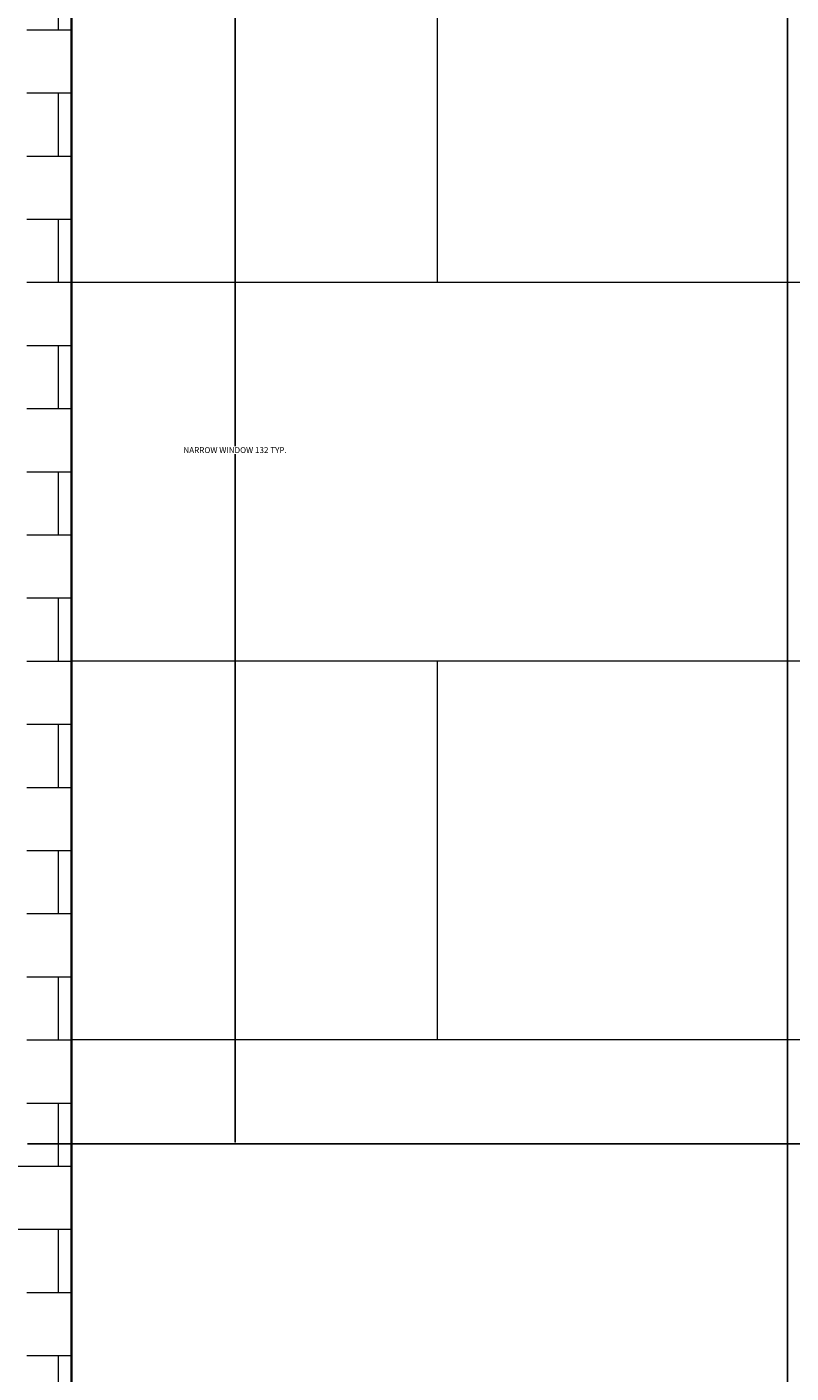
# Model space of a CAD drawing. Units: inches. Extents: x -26 to 776, y -22 to 650.
# Tile 24 of 62: x 285 to 358, y 292 to 420. Entities that reach past the tile are written whole.
import ezdxf

# ---------------------------------------------------------------- set-up
doc = ezdxf.new("R2010")
doc.units = ezdxf.units.IN
doc.header["$MEASUREMENT"] = 0
for name, color, linetype, lineweight in [('A-ANNO-DIMS', 2, 'Continuous', 18), ('A-WALL', 7, 'Continuous', 35), ('A-WALL-PATT', 8, 'Continuous', 13)]:
    doc.layers.add(name, color=color, linetype=linetype, lineweight=lineweight)
doc.styles.get("Standard").update_dxf_attribs({"font": 'arial.ttf'})
doc.dimstyles.get("Standard").update_dxf_attribs({"dimtxt": 0.5625, "dimasz": 0.18, "dimexe": 0.18, "dimexo": 0.0625, "dimgap": 0.09, "dimtad": 0, "dimtih": 1, "dimtoh": 1, "dimdec": 4, "dimzin": 0, "dimdsep": 46, "dimlunit": 4, "dimtxsty": 'Standard', "dimcen": 0.09, "dimadec": 0, "dimazin": 0, "dimtfac": 1, "dimtdec": 4, "dimtofl": 0, "dimtmove": 0, "dimatfit": 3, "dimfxl": 1, "dimtolj": 1, "dimtzin": 0, "dimarcsym": 0})

# ---------------------------------------------------------------- blocks, each defined once
blk = doc.blocks.new('*D9')
at = {"layer": 'A-ANNO-DIMS', "color": 0, "lineweight": -2, "transparency": 16777216}
for p, q in [((285.08, 446.01), (304.98, 446.01)), ((304.8, 445.83), (304.8, 380.44)), ((304.8, 314.3), (304.8, 379.68)), ((285.08, 314.12), (304.98, 314.12))]:
    blk.add_line(p, q, dxfattribs=at)
at = {"layer": 'A-ANNO-DIMS', "color": 0, "transparency": 16777216}
for points in [[(304.77, 445.83), (304.83, 445.83), (304.8, 446.01)], [(304.77, 314.3), (304.83, 314.3), (304.8, 314.12)]]:
    blk.add_solid(points, dxfattribs=at)
at = {"layer": 'Defpoints', "color": 0, "transparency": 16777216}
for p in [(285.02, 446.01), (304.8, 446.01), (285.02, 314.12)]:
    blk.add_point(p, dxfattribs=at)
at = {"layer": 'A-ANNO-DIMS', "color": 0, "transparency": 16777216, "insert": (304.8, 380.06), "char_height": 0.5625, "attachment_point": 5}
blk.add_mtext('\\A1;NARROW WINDOW 132 TYP.', dxfattribs=at)
blk = doc.blocks.new('*D28')
at = {"layer": 'A-ANNO-DIMS', "color": 0, "lineweight": -2, "transparency": 16777216}
for p, q in [((285.08, 314.12), (775.34, 314.12)), ((775.16, 313.94), (775.16, 243.14)), ((775.16, 171.6), (775.16, 242.4)), ((285.08, 171.42), (775.34, 171.42))]:
    blk.add_line(p, q, dxfattribs=at)
at = {"layer": 'A-ANNO-DIMS', "color": 0, "transparency": 16777216}
for points in [[(775.13, 313.94), (775.19, 313.94), (775.16, 314.12)], [(775.13, 171.6), (775.19, 171.6), (775.16, 171.42)]]:
    blk.add_solid(points, dxfattribs=at)
at = {"layer": 'Defpoints', "color": 0, "transparency": 16777216}
for p in [(285.02, 314.12), (775.16, 314.12), (285.02, 171.42)]:
    blk.add_point(p, dxfattribs=at)
at = {"layer": 'A-ANNO-DIMS', "color": 0, "transparency": 16777216, "insert": (775.16, 242.77), "char_height": 0.562, "attachment_point": 5}
blk.add_mtext('\\A1;142.7', dxfattribs=at)
blk = doc.blocks.new('*D34')
at = {"layer": 'A-ANNO-DIMS', "color": 0, "lineweight": -2, "transparency": 16777216}
for p, q in [((228.57, 528.3), (228.57, -21.31)), ((357.3, 528.36), (357.3, -21.31)), ((228.75, -21.13), (291.71, -21.13)), ((357.12, -21.13), (294.17, -21.13))]:
    blk.add_line(p, q, dxfattribs=at)
at = {"layer": 'A-ANNO-DIMS', "color": 0, "transparency": 16777216}
for points in [[(228.75, -21.1), (228.75, -21.16), (228.57, -21.13)], [(357.12, -21.1), (357.12, -21.16), (357.3, -21.13)]]:
    blk.add_solid(points, dxfattribs=at)
at = {"layer": 'Defpoints', "color": 0, "transparency": 16777216}
for p in [(357.3, 528.42), (228.57, 528.36), (357.3, -21.13)]:
    blk.add_point(p, dxfattribs=at)
at = {"layer": 'A-ANNO-DIMS', "color": 0, "transparency": 16777216, "insert": (292.94, -21.13), "char_height": 0.562, "attachment_point": 5}
blk.add_mtext('\\A1;128.73', dxfattribs=at)
blk = doc.blocks.new('*D39')
at = {"layer": 'A-ANNO-DIMS', "color": 0, "lineweight": -2, "transparency": 16777216}
for p, q in [((289.24, 15.54), (289.24, 649.86)), ((289.42, 649.68), (356.48, 649.68)), ((425.56, 649.68), (358.51, 649.68)), ((425.74, 15.54), (425.74, 649.86))]:
    blk.add_line(p, q, dxfattribs=at)
at = {"layer": 'A-ANNO-DIMS', "color": 0, "transparency": 16777216}
for points in [[(289.42, 649.71), (289.42, 649.65), (289.24, 649.68)], [(425.56, 649.71), (425.56, 649.65), (425.74, 649.68)]]:
    blk.add_solid(points, dxfattribs=at)
at = {"layer": 'Defpoints', "color": 0, "transparency": 16777216}
for p in [(425.74, 649.68), (289.24, 15.48), (425.74, 15.48)]:
    blk.add_point(p, dxfattribs=at)
at = {"layer": 'A-ANNO-DIMS', "color": 0, "transparency": 16777216, "insert": (357.49, 649.68), "char_height": 0.562, "attachment_point": 5}
blk.add_mtext('\\A1;136.5', dxfattribs=at)

msp = doc.modelspace()

# ---------------------------------------------------------------- hatches: boundary and pattern name
at = {"layer": 'A-WALL-PATT'}
h = msp.add_hatch(dxfattribs=at)
h.set_pattern_fill('AR-B816', color=256, scale=0.75)
h.paths.add_polyline_path([(289.2424, 504.4205), (231.4249, 504.4205), (231.4249, 458.1203), (231.4249, 221.6413), (231.4249, 209.6413), (231.4249, 159.4824), (285.0179, 159.4824), (285.0179, 171.4173), (236.4647, 171.4173), (236.4647, 294.4171), (236.4647, 303.3046), (285.0179, 303.3046), (285.0179, 294.4171), (285.0179, 171.4173), (285.0179, 159.4824), (289.2424, 159.4824), (289.2424, 291.1798), (289.2424, 458.1203)])
h.paths.add_polyline_path([(285.0179, 446.0063), (285.0179, 437.1188), (285.0179, 314.119), (236.4647, 314.119), (236.4647, 437.1188), (236.4647, 446.0063)], flags=16)
h = msp.add_hatch(dxfattribs=at)
h.set_pattern_fill('AR-B816', color=256, scale=4.5)
h.paths.add_polyline_path([(425.7434, 448.2114), (289.2424, 496.9554), (289.2424, 458.1203), (289.2424, 291.1798), (289.2424, 20.7937), (425.7434, 20.7937), (425.7434, 283.2492)])

# ---------------------------------------------------------------- linework, layer by layer
at = {"layer": 'A-WALL'}
msp.add_line((289.2424, 458.1203), (289.2424, 291.1798), dxfattribs=at)

# ---------------------------------------------------------------- dimensions: what is measured, and where the dimension line sits
at = {"layer": 'A-ANNO-DIMS'}
for base, p1, p2, override, picture, middle in [((425.7434, 649.6763), (289.2424, 15.4824), (425.7434, 15.4824), {"dimdec": 1, "dimlfac": 1, "dimrnd": 0, "dimzin": 0, "dimdsep": 46, "dimlunit": 2}, '*D39', (357.4929, 649.6763)), ((357.3034, -21.1349), (228.5733, 528.3585), (357.3034, 528.4233), {"dimdec": 2, "dimlfac": 1, "dimrnd": 0, "dimzin": 0, "dimdsep": 46, "dimlunit": 2}, '*D34', (292.9384, -21.1349))]:
    dim = msp.add_linear_dim(base=base, p1=p1, p2=p2, dimstyle='Standard', override=override, dxfattribs=at)
    dim.commit()
    dim.dimension.update_dxf_attribs({"geometry": picture, "text_midpoint": middle})
dim = msp.add_linear_dim(base=(304.801, 446.0063), p1=(285.0179, 314.119), p2=(285.0179, 446.0063), angle=90, text='NARROW WINDOW <> TYP.', dimstyle='Standard', override={"dimdec": 0, "dimlfac": 1, "dimrnd": 0, "dimzin": 0, "dimdsep": 46, "dimlunit": 2}, dxfattribs=at)
dim.commit()
dim.dimension.update_dxf_attribs({"geometry": '*D9', "text_midpoint": (304.801, 380.0626)})
dim = msp.add_linear_dim(base=(775.1553, 314.119), p1=(285.0179, 171.4173), p2=(285.0179, 314.119), angle=90, dimstyle='Standard', override={"dimdec": 1, "dimlfac": 1, "dimrnd": 0, "dimzin": 0, "dimdsep": 46, "dimlunit": 2}, dxfattribs=at)
dim.commit()
dim.dimension.update_dxf_attribs({"geometry": '*D28', "text_midpoint": (775.1553, 242.7682)})

doc.saveas('drawing.dxf')
